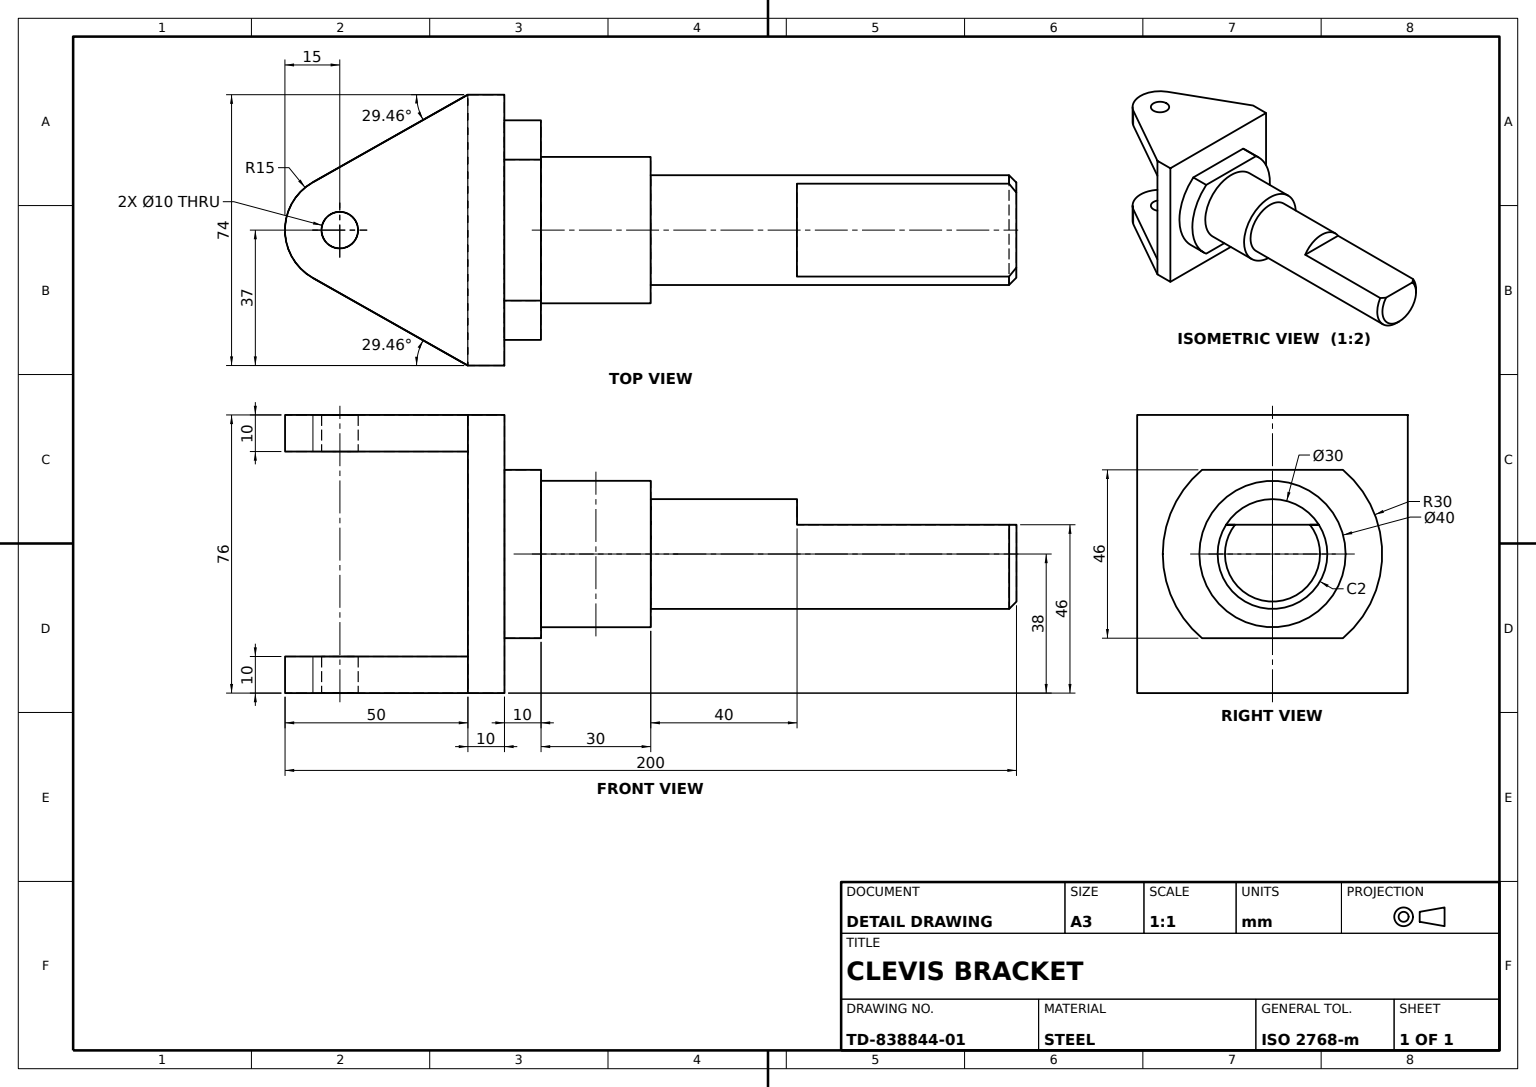
from build123d import *

# Parameters (mm, degrees)
BASE_PLATE_SKETCH_W         = 10
BASE_PLATE_SKETCH_H         = 76
BASE_PLATE_DEPTH            = 74
FORK_EAR_1_DEPTH            = 10
FORK_START                  = -10
FORK_EAR_2_DEPTH            = 10
PIVOT_PIN_HOLE_SKETCH_R     = 5
PIVOT_PIN_HOLE_10_DEPTH     = 100
HEX_COLLAR_DEPTH            = 10
SHOULDER_40_SKETCH_R        = 20
SHOULDER_40_DEPTH           = 30
SHAFT_30_SKETCH_R           = 15
SHAFT_30_DEPTH              = 100
SHAFT_START                 = -60
SHAFT_FLAT_DEPTH            = 60
SHAFT_END_CHAMFER_2X45_SIZE = 2


with BuildPart() as part:
    # Base Plate Sketch → Base Plate (new body)
    with BuildSketch(Plane.XY):
        with Locations((-5, 0)):
            Rectangle(BASE_PLATE_SKETCH_W, BASE_PLATE_SKETCH_H)
    extrude(amount=-BASE_PLATE_DEPTH)

    # Fork Ear 1 Sketch → Fork Ear 1 (add)
    with BuildSketch(Plane(origin=(0, 38, 0), x_dir=(1, 0, 0), z_dir=(0, 1, 0))):
        with BuildLine():
            Line((-10, 74), (-10, 0))
            Line((-10, 0), (-52.377859531, 23.939862606))
            ThreePointArc((-52.377859531, 23.939862606), (-60, 37), (-52.377859531, 50.060137394))
            Line((-52.377859531, 50.060137394), (-10, 74))
        make_face()
    extrude(amount=-FORK_EAR_1_DEPTH)

    # Fork Ear 2 Sketch → Fork Ear 2 (add)
    with BuildSketch(Plane.XZ.offset(38).offset(FORK_START)):
        with BuildLine():
            Line((-52.377859531, -23.939862606), (-10, 0))
            Line((-10, 0), (-10, -74))
            Line((-10, -74), (-52.377859531, -50.060137394))
            ThreePointArc((-52.377859531, -50.060137394), (-60, -37), (-52.377859531, -23.939862606))
        make_face()
    extrude(amount=FORK_EAR_2_DEPTH)

    # Pivot Pin Hole Sketch → Pivot Pin Hole Ø10 (cut)
    with BuildSketch(Plane.XZ.offset(38)):
        with Locations(Location((-45, -37, 0), (0, 0, 270))):
            Circle(PIVOT_PIN_HOLE_SKETCH_R)
    extrude(amount=-PIVOT_PIN_HOLE_10_DEPTH, mode=Mode.SUBTRACT)

    # Hex Collar Sketch → Hex Collar (add)
    with BuildSketch(Plane(origin=(0, 0, 0), x_dir=(0, 0, -1), z_dir=(1, 0, 0))):
        with BuildLine():
            Line((17.738639716, 23), (56.261360284, 23))
            ThreePointArc((56.261360284, 23), (67, 0), (56.261360284, -23))
            Line((56.261360284, -23), (17.738639716, -23))
            ThreePointArc((17.738639716, -23), (7, 0), (17.738639716, 23))
        make_face()
    extrude(amount=HEX_COLLAR_DEPTH)

    # Shoulder Ø40 Sketch → Shoulder Ø40 (add)
    with BuildSketch(Plane(origin=(10, 0, 0), x_dir=(0, 0, -1), z_dir=(1, 0, 0))):
        with Locations((37, 0)):
            Circle(SHOULDER_40_SKETCH_R)
    extrude(amount=SHOULDER_40_DEPTH)

    # Shaft Ø30 Sketch → Shaft Ø30 (add)
    with BuildSketch(Plane(origin=(40, 0, 0), x_dir=(0, 0, -1), z_dir=(1, 0, 0))):
        with Locations((37, 0)):
            Circle(SHAFT_30_SKETCH_R)
    extrude(amount=SHAFT_30_DEPTH)

    # Shaft Flat Sketch → Shaft Flat (cut)
    with BuildSketch(Plane(origin=(140, 0, 0), x_dir=(0, 0, -1), z_dir=(1, 0, 0)).offset(SHAFT_START)):
        with BuildLine():
            Line((24.31142246, 8), (49.68857754, 8))
            ThreePointArc((49.68857754, 8), (37, 15), (24.31142246, 8))
        make_face()
    extrude(amount=SHAFT_FLAT_DEPTH, mode=Mode.SUBTRACT)

    # Shaft End Chamfer 2x45°
    shaft_end_chamfer_2x45_edges = [part.edges().sort_by_distance(p)[0] for p in [
        (140, -14.410563193, -32.836387572),
    ]]
    chamfer(shaft_end_chamfer_2x45_edges, length=SHAFT_END_CHAMFER_2X45_SIZE)


solid = part.part
